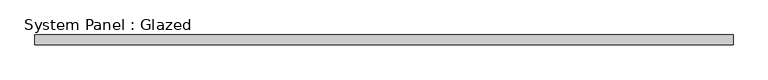
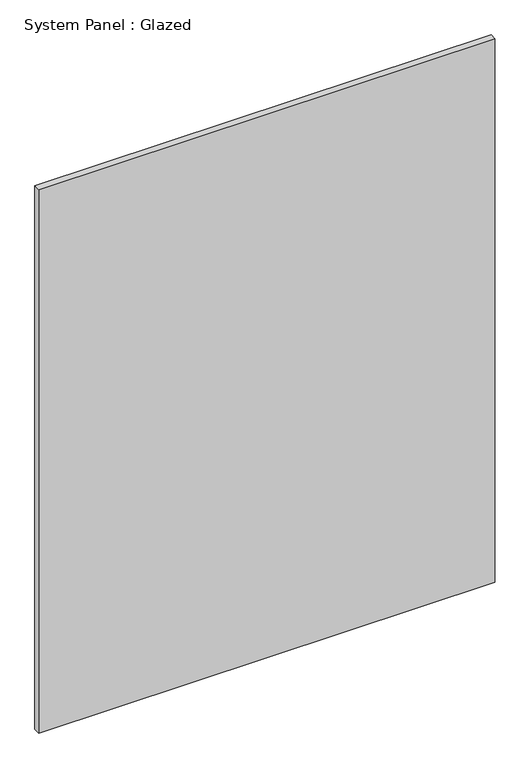
"""IFC4 building model written with IfcOpenShell, lengths in millimetres: plate geometry, System Panel : Glazed."""

from ifc_helpers import new_model, si_unit, origin, origin_with_axes, place, context, project, spatial, polyline, outline, extrude, source, transform, mapped, element, save


def system_panel_glazed_98faf640(model_context):
    return source(origin(), model_context, "Body", "SweptSolid", [
        extrude(outline(polyline([(917.575, 19.05), (-917.575, 19.05), (-917.575, 44.45), (917.575, 44.45), (917.575, 19.05)])), origin_with_axes(), (0.0, 0.0, 1.0), 2311.4),
    ])


if __name__ == "__main__":
    model = new_model("IFC4")
    model_context = context("Model", 3, world=origin())
    ifc_project = project(units=[si_unit("LENGTHUNIT", "METRE", prefix="MILLI")], contexts=[model_context])
    site = spatial("IfcSite", under=ifc_project)
    building = spatial("IfcBuilding", under=site)
    placement = place(None, origin())
    system_panel_glazed_shape = system_panel_glazed_98faf640(model_context)
    element("IfcPlate", 1, ObjectType="System Panel : Glazed", at=placement, inside=building, context=model_context, shape_type="MappedRepresentation", body=[
        mapped(system_panel_glazed_shape, transform((0.0, 0.0, 0.0), x_axis=(1.0, 0.0, 0.0), y_axis=(0.0, 1.0, 0.0), z_axis=(0.0, 0.0, 1.0))),
    ])
    save(model, "model.ifc")

# Revit data of these elements
# Type "System Panel : Glazed"
#   Construction Type Id = "GSP4R"
#   Analytic Construction = "1/8 in Pilkington single glazing"
#   Visual Light Transmittance = 0.9
#   Solar Heat Gain Coefficient = 0.86
#   Heat Transfer Coefficient (U) = 1.18115 BTU/(h·ft²·°F)
# Element 1 (IfcPlate, "System Panel : Glazed")
#   Materials on its faces: "Glass"
# Materials
#   "Glass": class "Glass", colour RGB 0 128 192, transparency 0.75, Description = "Soda Lime Glass", Cost = 0
